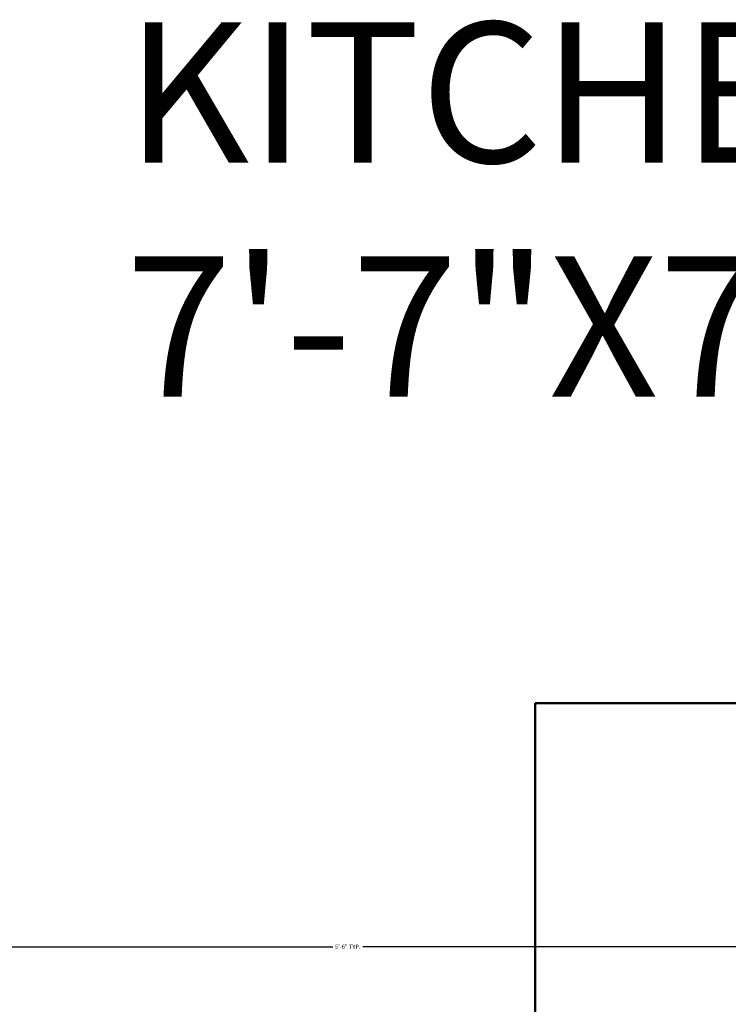
# Model space of a CAD drawing. Units: inches. Extents: x -173 to 545, y -746 to 104.
# Tile 25 of 32: x 189 to 219, y -94 to -52. Entities that reach past the tile are written whole.
import ezdxf

# ---------------------------------------------------------------- set-up
doc = ezdxf.new("R2010")
doc.units = ezdxf.units.IN
doc.header["$MEASUREMENT"] = 0
for name, color, linetype, lineweight in [('A-ANNO-DIMS', 2, 'Continuous', 18), ('A-AREA-IDEN', 7, 'Continuous', 18), ('A-WALL', 7, 'Continuous', 50)]:
    doc.layers.add(name, color=color, linetype=linetype, lineweight=lineweight)
doc.styles.get("Standard").update_dxf_attribs({"font": 'arial.ttf'})
doc.dimstyles.get("Standard").update_dxf_attribs({"dimtxt": 0.18, "dimasz": 0.18, "dimexe": 0.18, "dimexo": 0.0625, "dimgap": 0.09, "dimtad": 0, "dimtih": 1, "dimtoh": 1, "dimdec": 0, "dimzin": 0, "dimdsep": 46, "dimlunit": 3, "dimtxsty": 'Standard', "dimcen": 0.09, "dimadec": 0, "dimazin": 0, "dimtfac": 1, "dimtdec": 0, "dimtofl": 0, "dimtmove": 0, "dimatfit": 3, "dimfxl": 1, "dimtolj": 1, "dimtzin": 0, "dimarcsym": 0})

# ---------------------------------------------------------------- blocks, each defined once
blk = doc.blocks.new('*D77')
at = {"layer": 'A-ANNO-DIMS', "color": 0, "lineweight": -2, "transparency": 16777216}
for p, q in [((169.801, -81.424), (169.801, -91.946)), ((235.801, -81.424), (235.801, -91.946)), ((169.981, -91.766), (202.163, -91.766)), ((235.621, -91.766), (203.44, -91.766))]:
    blk.add_line(p, q, dxfattribs=at)
at = {"layer": 'A-ANNO-DIMS', "color": 0, "transparency": 16777216}
for points in [[(169.981, -91.736), (169.981, -91.796), (169.801, -91.766)], [(235.621, -91.736), (235.621, -91.796), (235.801, -91.766)]]:
    blk.add_solid(points, dxfattribs=at)
at = {"layer": 'Defpoints', "color": 0, "transparency": 16777216}
for p in [(169.801, -81.362), (235.801, -81.362), (235.801, -91.766)]:
    blk.add_point(p, dxfattribs=at)
at = {"layer": 'A-ANNO-DIMS', "color": 0, "transparency": 16777216, "insert": (202.801, -91.766), "char_height": 0.18, "attachment_point": 5}
blk.add_mtext('\\A1;5\'-6" TYP.', dxfattribs=at)

msp = doc.modelspace()

# ---------------------------------------------------------------- linework, layer by layer
at = {"layer": 'A-WALL'}
for q in [(260.801, -81.362), (210.801, -128.862)]:
    msp.add_line((210.801, -81.362), q, dxfattribs=at)

# ---------------------------------------------------------------- texts
at = {"layer": 'A-AREA-IDEN', "insert": (193.303, -52.27), "char_height": 6, "attachment_point": 1}
msp.add_mtext('KITCHEN\\P7\'-7"X7\'-5"', dxfattribs=at)

# ---------------------------------------------------------------- dimensions: what is measured, and where the dimension line sits
at = {"layer": 'A-ANNO-DIMS'}
dim = msp.add_linear_dim(base=(235.801, -91.766), p1=(169.801, -81.362), p2=(235.801, -81.362), text='<> TYP.', dimstyle='Standard', override={"dimdec": 1, "dimlfac": 1, "dimrnd": 0, "dimzin": 1, "dimdsep": 46, "dimlunit": 4, "dimfrac": 2}, dxfattribs=at)
dim.commit()
dim.dimension.update_dxf_attribs({"geometry": '*D77', "text_midpoint": (202.801, -91.766)})

doc.saveas('drawing.dxf')
